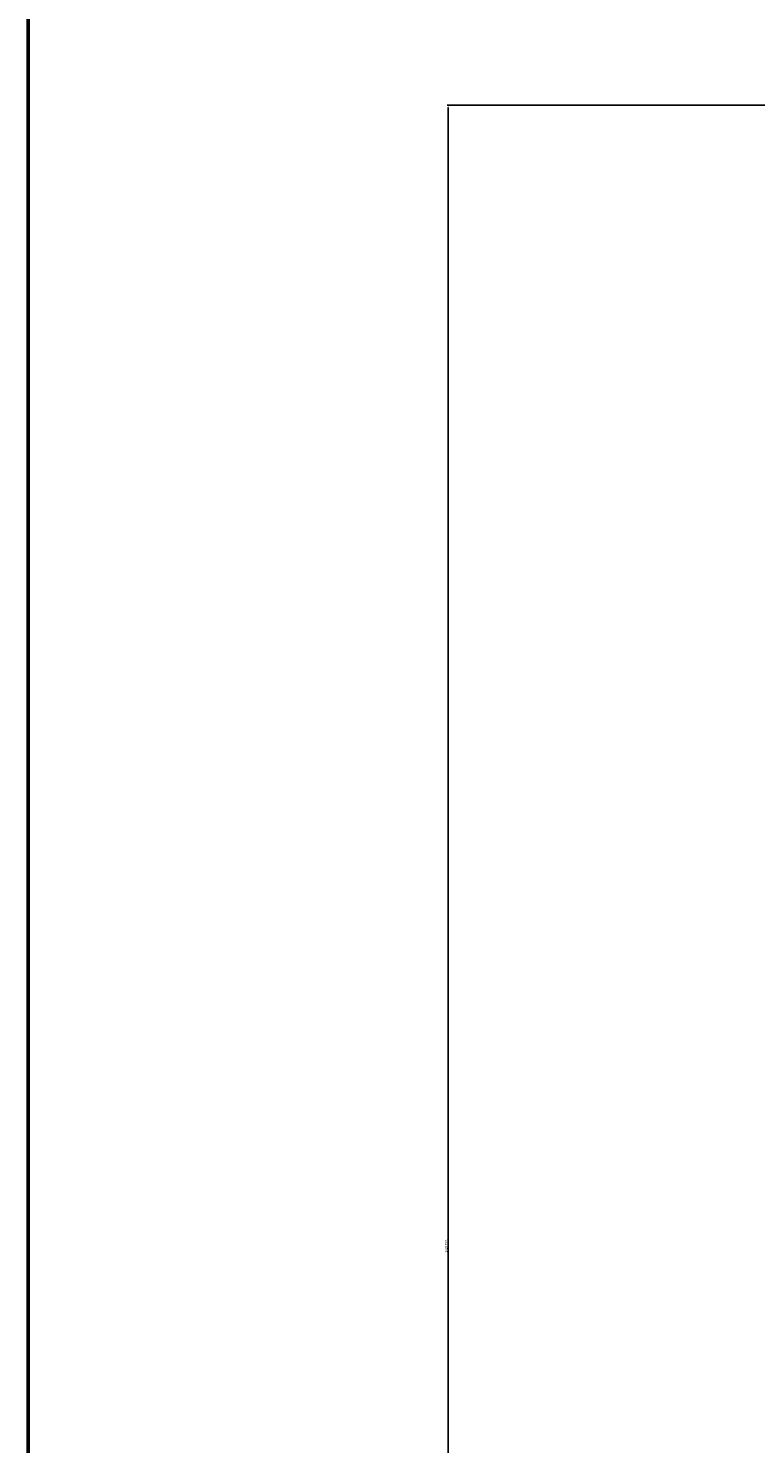
# Model space of a CAD drawing. Units: millimetres. Extents: x -857 to 54106, y -13666 to 13947.
# Tile 27 of 41: x 30020 to 30856, y 9552 to 11178. Entities that reach past the tile are written whole.
import ezdxf

# ---------------------------------------------------------------- set-up
doc = ezdxf.new("R2010")
doc.units = ezdxf.units.MM
doc.layers.add('A-ANNO-DIMS', color=2, linetype='Continuous', lineweight=18)
doc.layers.add('A-WALL', color=7, linetype='Continuous', lineweight=50)
doc.styles.get("Standard").update_dxf_attribs({"font": 'arial.ttf'})
doc.dimstyles.new('ISO-25', dxfattribs={"dimtxt": 2.5, "dimasz": 2.5, "dimexe": 1.25, "dimexo": 0.625, "dimtad": 1, "dimtxsty": 'Standard', "dimcen": 2.5, "dimadec": 0, "dimazin": 0, "dimtfac": 1, "dimtmove": 0, "dimatfit": 3, "dimfxl": 1, "dimarcsym": 0})

# ---------------------------------------------------------------- blocks, each defined once
blk = doc.blocks.new('*D48')
at = {"layer": 'A-ANNO-DIMS', "color": 0, "lineweight": -2, "transparency": 16777216}
for p, q in [((30908.6, 11089.5), (30501.4, 11089.5)), ((30502.6, 11087), (30502.6, 8471.5)), ((30908.6, 8469), (30501.4, 8469))]:
    blk.add_line(p, q, dxfattribs=at)
at = {"layer": 'A-ANNO-DIMS', "color": 0, "transparency": 16777216}
for points in [[(30502.2, 11087), (30503, 11087), (30502.6, 11089.5)], [(30502.2, 8471.5), (30503, 8471.5), (30502.6, 8469)]]:
    blk.add_solid(points, dxfattribs=at)
at = {"layer": 'Defpoints', "color": 0, "transparency": 16777216}
for p in [(30909.3, 11089.5), (30502.6, 8469), (30909.3, 8469)]:
    blk.add_point(p, dxfattribs=at)
at = {"layer": 'A-ANNO-DIMS', "color": 0, "transparency": 16777216, "insert": (30500.7, 9779.2), "char_height": 2.5, "attachment_point": 5, "rotation": 90}
blk.add_mtext('2620 TYP.', dxfattribs=at)

msp = doc.modelspace()

# ---------------------------------------------------------------- linework, layer by layer
at = {"layer": 'A-WALL'}
msp.add_line((30020.079, 11404.231), (30020.079, 9184.795), dxfattribs=at)

# ---------------------------------------------------------------- dimensions: what is measured, and where the dimension line sits
at = {"layer": 'A-ANNO-DIMS'}
dim = msp.add_linear_dim(base=(30502.63, 8468.999), p1=(30909.254, 11089.463), p2=(30909.254, 8468.999), angle=270, text='<> TYP.', dimstyle='ISO-25', override={"dimdec": 0, "dimrnd": 0, "dimzin": 0, "dimlunit": 2}, dxfattribs=at)
dim.commit()
dim.dimension.update_dxf_attribs({"geometry": '*D48', "text_midpoint": (30500.728, 9779.231)})

doc.saveas('drawing.dxf')
